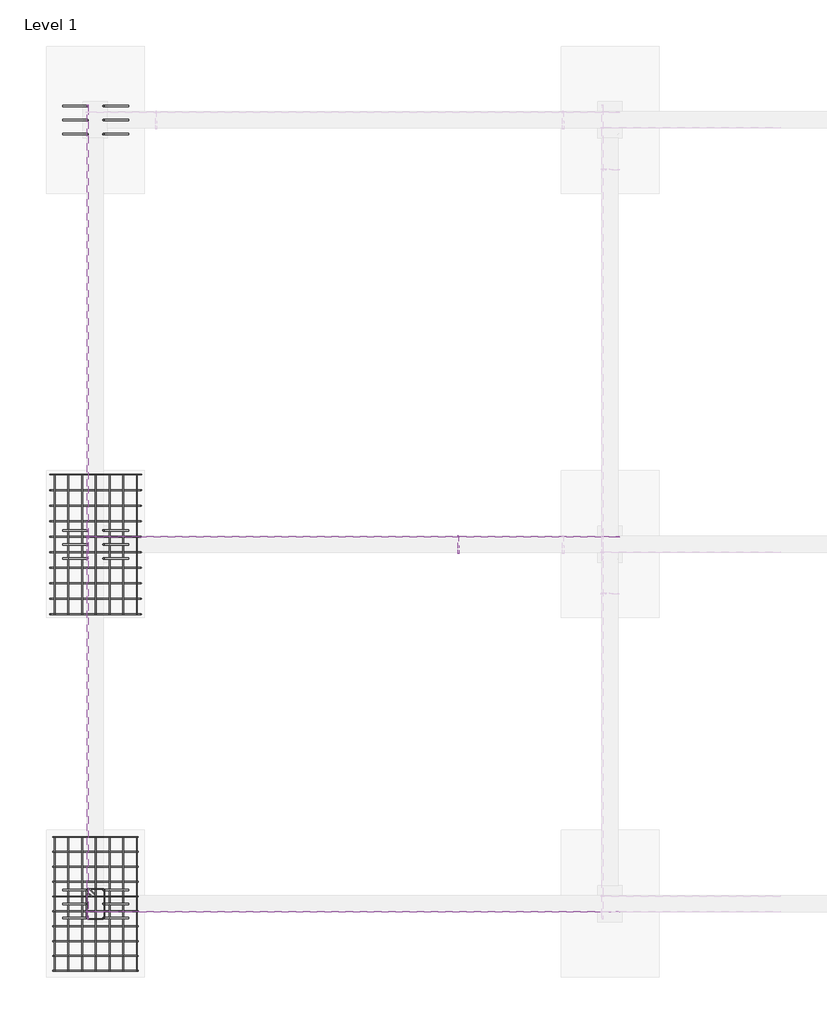
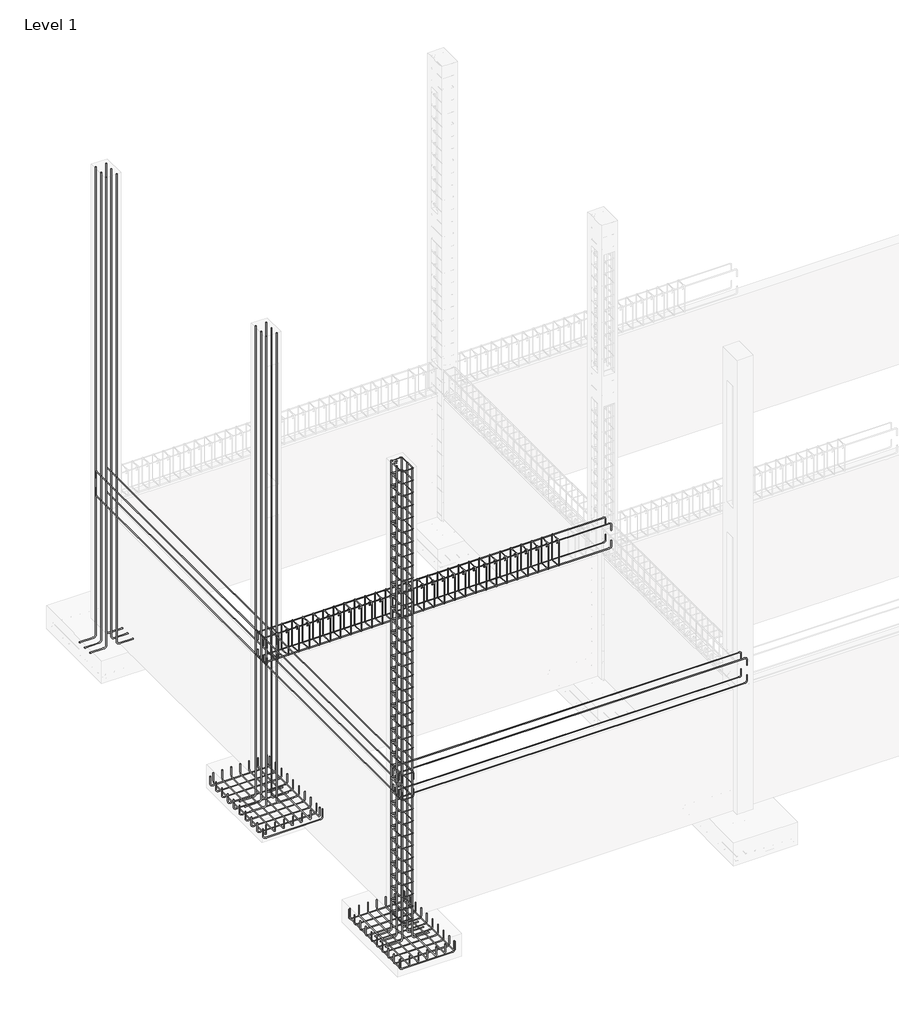
# One storey, part 3 of 8: 20 reinforcing bars.
"""IFC4 building model written with IfcOpenShell, lengths in millimetres."""

from ifc_helpers import new_model, si_unit, point, frame, origin, place, context, project, spatial, polyline, circle_curve, trimmed, segment, composite_curve, source, transform, mapped, element, save
from ifc_brep_helpers import swept_disk

model = new_model("IFC4")

# Units and contexts
model_context = context("Model", 3, world=origin())
ifc_project = project(units=[si_unit("LENGTHUNIT", "METRE", prefix="MILLI")], contexts=[model_context])

# Site, building, storey
site = spatial("IfcSite", under=ifc_project)
building = spatial("IfcBuilding", under=site)
storey = spatial("IfcBuildingStorey", under=building, Name="Level 1", Elevation=0.0)

# Reinforcing bars
placement = place(None, origin())
reinforcing_bar_shape = source(origin(), model_context, "Body", "SolidModel", [
    swept_disk(composite_curve([segment(polyline([(-20238.7033089, 3954.7360327, -178.562), (-20238.7033089, 3954.7360327, -330.962)]), True, "CONTINUOUS"), segment(trimmed(circle_curve(frame((-20282.7723089, 3954.7360327, -330.962), z_axis=(0.0, 1.0, 0.0), x_axis=(44.068999999999505, 0.0, 0.0)), 44.069), [point((-20238.7033089, 3954.7360327, -330.962))], [point((-20282.7723089, 3954.7360327, -375.031))], True, "CARTESIAN"), True, "CONTINUOUS"), segment(polyline([(-20282.7723089, 3954.7360327, -375.031), (-21249.4963089, 3954.7360327, -375.031)]), True, "CONTINUOUS"), segment(trimmed(circle_curve(frame((-21249.4963089, 3954.7360327, -330.962), z_axis=(0.0, 1.0, 0.0), x_axis=(0.0, 0.0, -44.06900000000002)), 44.069), [point((-21249.4963089, 3954.7360327, -375.031))], [point((-21293.5653089, 3954.7360327, -330.962))], True, "CARTESIAN"), True, "CONTINUOUS"), segment(polyline([(-21293.5653089, 3954.7360327, -330.962), (-21293.5653089, 3954.7360327, -178.562)]), True, "CONTINUOUS")], self_intersect=False), 5.969),
])
element("IfcReinforcingBar", 1, at=placement, inside=storey, context=model_context, shape_type="MappedRepresentation", body=[
    mapped(reinforcing_bar_shape, transform((0.0, 0.0, 0.0), x_axis=(1.0, 0.0, 0.0), y_axis=(0.0, 1.0, 0.0), z_axis=(0.0, 0.0, 1.0))),
    mapped(reinforcing_bar_shape, transform((0.0, -184.9402222, 0.0), x_axis=(1.0, 0.0, 0.0), y_axis=(0.0, 1.0, 0.0), z_axis=(0.0, 0.0, 1.0))),
    mapped(reinforcing_bar_shape, transform((0.0, -369.8804444, 0.0), x_axis=(1.0, 0.0, 0.0), y_axis=(0.0, 1.0, 0.0), z_axis=(0.0, 0.0, 1.0))),
    mapped(reinforcing_bar_shape, transform((0.0, -554.8206667, 0.0), x_axis=(1.0, 0.0, 0.0), y_axis=(0.0, 1.0, 0.0), z_axis=(0.0, 0.0, 1.0))),
    mapped(reinforcing_bar_shape, transform((0.0, -739.7608889, 0.0), x_axis=(1.0, 0.0, 0.0), y_axis=(0.0, 1.0, 0.0), z_axis=(0.0, 0.0, 1.0))),
    mapped(reinforcing_bar_shape, transform((0.0, -924.7011111, 0.0), x_axis=(1.0, 0.0, 0.0), y_axis=(0.0, 1.0, 0.0), z_axis=(0.0, 0.0, 1.0))),
    mapped(reinforcing_bar_shape, transform((0.0, -1109.6413333, 0.0), x_axis=(1.0, 0.0, 0.0), y_axis=(0.0, 1.0, 0.0), z_axis=(0.0, 0.0, 1.0))),
    mapped(reinforcing_bar_shape, transform((0.0, -1294.5815556, 0.0), x_axis=(1.0, 0.0, 0.0), y_axis=(0.0, 1.0, 0.0), z_axis=(0.0, 0.0, 1.0))),
    mapped(reinforcing_bar_shape, transform((0.0, -1479.5217778, 0.0), x_axis=(1.0, 0.0, 0.0), y_axis=(0.0, 1.0, 0.0), z_axis=(0.0, 0.0, 1.0))),
    mapped(reinforcing_bar_shape, transform((0.0, -1664.462, 0.0), x_axis=(1.0, 0.0, 0.0), y_axis=(0.0, 1.0, 0.0), z_axis=(0.0, 0.0, 1.0))),
])
reinforcing_bar_2_shape = source(origin(), model_context, "Body", "SolidModel", [
    swept_disk(composite_curve([segment(polyline([(-21274.1343089, 3954.7360327, -165.481), (-21274.1343089, 3954.7360327, -317.881)]), True, "CONTINUOUS"), segment(trimmed(circle_curve(frame((-21274.1343089, 3910.6670327, -317.881), z_axis=(-1.0, 0.0, 0.0), x_axis=(0.0, 44.06899999999996, 0.0)), 44.069), [point((-21274.1343089, 3954.7360327, -317.881))], [point((-21274.1343089, 3910.6670327, -361.95))], True, "CARTESIAN"), True, "CONTINUOUS"), segment(polyline([(-21274.1343089, 3910.6670327, -361.95), (-21274.1343089, 2334.3430327, -361.95)]), True, "CONTINUOUS"), segment(trimmed(circle_curve(frame((-21274.1343089, 2334.3430327, -317.881), z_axis=(-1.0, 0.0, 0.0), x_axis=(0.0, 0.0, -44.06900000000002)), 44.069), [point((-21274.1343089, 2334.3430327, -361.95))], [point((-21274.1343089, 2290.2740327, -317.881))], True, "CARTESIAN"), True, "CONTINUOUS"), segment(polyline([(-21274.1343089, 2290.2740327, -317.881), (-21274.1343089, 2290.2740327, -165.481)]), True, "CONTINUOUS")], self_intersect=False), 5.969),
])
element("IfcReinforcingBar", 2, at=placement, inside=storey, context=model_context, shape_type="MappedRepresentation", body=[
    mapped(reinforcing_bar_2_shape, transform((0.0, 0.0, 0.0), x_axis=(1.0, 0.0, 0.0), y_axis=(0.0, 1.0, 0.0), z_axis=(0.0, 0.0, 1.0))),
    mapped(reinforcing_bar_2_shape, transform((170.5954914, 0.0, 0.0), x_axis=(1.0, 0.0, 0.0), y_axis=(0.0, 1.0, 0.0), z_axis=(0.0, 0.0, 1.0))),
    mapped(reinforcing_bar_2_shape, transform((341.1909829, 0.0, 0.0), x_axis=(1.0, 0.0, 0.0), y_axis=(0.0, 1.0, 0.0), z_axis=(0.0, 0.0, 1.0))),
    mapped(reinforcing_bar_2_shape, transform((511.7864743, 0.0, 0.0), x_axis=(1.0, 0.0, 0.0), y_axis=(0.0, 1.0, 0.0), z_axis=(0.0, 0.0, 1.0))),
    mapped(reinforcing_bar_2_shape, transform((682.3819658, 0.0, 0.0), x_axis=(1.0, 0.0, 0.0), y_axis=(0.0, 1.0, 0.0), z_axis=(0.0, 0.0, 1.0))),
    mapped(reinforcing_bar_2_shape, transform((852.9774572, 0.0, 0.0), x_axis=(1.0, 0.0, 0.0), y_axis=(0.0, 1.0, 0.0), z_axis=(0.0, 0.0, 1.0))),
    mapped(reinforcing_bar_2_shape, transform((1023.5729487, 0.0, 0.0), x_axis=(1.0, 0.0, 0.0), y_axis=(0.0, 1.0, 0.0), z_axis=(0.0, 0.0, 1.0))),
])
reinforcing_bar_3_shape = source(origin(), model_context, "Body", "SolidModel", [
    swept_disk(composite_curve([segment(polyline([(-20667.7093089, 3297.1300327, 9105.9), (-20667.7093089, 3297.1300327, -307.9115)]), True, "CONTINUOUS"), segment(trimmed(circle_curve(frame((-20621.6083089, 3297.1300327, -307.9115), z_axis=(0.0, -1.0, 0.0), x_axis=(-46.10100000000239, 0.0, 0.0)), 46.101), [point((-20667.7093089, 3297.1300327, -307.9115))], [point((-20621.6083089, 3297.1300327, -354.0125))], True, "CARTESIAN"), True, "CONTINUOUS"), segment(polyline([(-20621.6083089, 3297.1300327, -354.0125), (-20355.0353089, 3297.1300327, -354.0125)]), True, "CONTINUOUS")], self_intersect=False), 8.001),
])
element("IfcReinforcingBar", 3, at=placement, inside=storey, context=model_context, shape_type="MappedRepresentation", body=[
    mapped(reinforcing_bar_3_shape, transform((0.0, 0.0, 0.0), x_axis=(1.0, 0.0, 0.0), y_axis=(0.0, 1.0, 0.0), z_axis=(0.0, 0.0, 1.0))),
    mapped(reinforcing_bar_3_shape, transform((0.0, -174.625, 0.0), x_axis=(1.0, 0.0, 0.0), y_axis=(0.0, 1.0, 0.0), z_axis=(0.0, 0.0, 1.0))),
    mapped(reinforcing_bar_3_shape, transform((0.0, -349.25, 0.0), x_axis=(1.0, 0.0, 0.0), y_axis=(0.0, 1.0, 0.0), z_axis=(0.0, 0.0, 1.0))),
])
reinforcing_bar_4_shape = source(origin(), model_context, "Body", "SolidModel", [
    swept_disk(composite_curve([segment(polyline([(-21177.2333089, 3297.1300327, -354.0125), (-20910.6603089, 3297.1300327, -354.0125)]), True, "CONTINUOUS"), segment(trimmed(circle_curve(frame((-20910.6603089, 3297.1300327, -307.9115), z_axis=(0.0, -1.0, 0.0), x_axis=(0.0, 0.0, -46.101)), 46.101), [point((-20910.6603089, 3297.1300327, -354.0125))], [point((-20864.5593089, 3297.1300327, -307.9115))], True, "CARTESIAN"), True, "CONTINUOUS"), segment(polyline([(-20864.5593089, 3297.1300327, -307.9115), (-20864.5593089, 3297.1300327, 9105.9)]), True, "CONTINUOUS")], self_intersect=False), 8.001),
])
element("IfcReinforcingBar", 4, at=placement, inside=storey, context=model_context, shape_type="MappedRepresentation", body=[
    mapped(reinforcing_bar_4_shape, transform((0.0, 0.0, 0.0), x_axis=(1.0, 0.0, 0.0), y_axis=(0.0, 1.0, 0.0), z_axis=(0.0, 0.0, 1.0))),
    mapped(reinforcing_bar_4_shape, transform((0.0, -174.625, 0.0), x_axis=(1.0, 0.0, 0.0), y_axis=(0.0, 1.0, 0.0), z_axis=(0.0, 0.0, 1.0))),
    mapped(reinforcing_bar_4_shape, transform((0.0, -349.25, 0.0), x_axis=(1.0, 0.0, 0.0), y_axis=(0.0, 1.0, 0.0), z_axis=(0.0, 0.0, 1.0))),
])
reinforcing_bar_5_shape = source(origin(), model_context, "Body", "SolidModel", [
    swept_disk(composite_curve([segment(polyline([(-20780.3918482, 3245.4710993, 42.037), (-20837.2560453, 3302.3352963, 42.037)]), True, "CONTINUOUS"), segment(trimmed(circle_curve(frame((-20853.5103089, 3286.0810327, 42.037), z_axis=(0.0, 0.0, 1.0), x_axis=(16.25426359999983, 16.254263600000286, 0.0)), 22.987), [point((-20837.2560453, 3302.3352963, 42.037))], [point((-20876.4973089, 3286.0810327, 42.037))], True, "CARTESIAN"), True, "CONTINUOUS"), segment(polyline([(-20876.4973089, 3286.0810327, 42.037), (-20876.4973089, 2958.9290327, 42.037)]), True, "CONTINUOUS"), segment(trimmed(circle_curve(frame((-20853.5103089, 2958.9290327, 42.037), z_axis=(0.0, 0.0, 1.0), x_axis=(-22.98700000000099, 0.0, 0.0)), 22.987), [point((-20876.4973089, 2958.9290327, 42.037))], [point((-20853.5103089, 2935.9420327, 42.037))], True, "CARTESIAN"), True, "CONTINUOUS"), segment(polyline([(-20853.5103089, 2935.9420327, 42.037), (-20678.7583089, 2935.9420327, 42.037)]), True, "CONTINUOUS"), segment(trimmed(circle_curve(frame((-20678.7583089, 2958.9239161, 41.5520181), z_axis=(0.0, 0.02109809375347505, 0.9997774104469302), x_axis=(0.0, -22.981883400000243, 0.4849819000000011)), 22.987), [point((-20678.7583089, 2935.9420327, 42.037))], [point((-20655.7713089, 2958.9239161, 41.5520181))], True, "CARTESIAN"), True, "CONTINUOUS"), segment(polyline([(-20655.7713089, 2958.9239161, 41.5520181), (-20655.7713089, 3286.0861494, 34.6479819)]), True, "CONTINUOUS"), segment(trimmed(circle_curve(frame((-20678.7583089, 3286.0861494, 34.6479819), z_axis=(0.0, 0.02109809375347505, 0.9997774104469302), x_axis=(22.98700000000099, 0.0, 0.0)), 22.987), [point((-20655.7713089, 3286.0861494, 34.6479819))], [point((-20678.7583089, 3309.0680327, 34.163))], True, "CARTESIAN"), True, "CONTINUOUS"), segment(polyline([(-20678.7583089, 3309.0680327, 34.163), (-20853.5103089, 3309.0680327, 34.163)]), True, "CONTINUOUS"), segment(trimmed(circle_curve(frame((-20853.5103089, 3286.0810327, 34.163), z_axis=(0.0, 0.0, 1.0), x_axis=(0.0, 22.98700000000008, 0.0)), 22.987), [point((-20853.5103089, 3309.0680327, 34.163))], [point((-20869.7645724, 3269.8267692, 34.163))], True, "CARTESIAN"), True, "CONTINUOUS"), segment(polyline([(-20869.7645724, 3269.8267692, 34.163), (-20812.9003754, 3212.9625721, 34.163)]), True, "CONTINUOUS")], self_intersect=False), 3.937),
])
element("IfcReinforcingBar", 5, at=placement, inside=storey, context=model_context, shape_type="MappedRepresentation", body=[
    mapped(reinforcing_bar_5_shape, transform((0.0, 0.0, 0.0), x_axis=(1.0, 0.0, 0.0), y_axis=(0.0, 1.0, 0.0), z_axis=(0.0, 0.0, 1.0))),
    mapped(reinforcing_bar_5_shape, transform((0.0, 0.0, 244.8628649), x_axis=(1.0, 0.0, 0.0), y_axis=(0.0, 1.0, 0.0), z_axis=(0.0, 0.0, 1.0))),
    mapped(reinforcing_bar_5_shape, transform((0.0, 0.0, 489.7257297), x_axis=(1.0, 0.0, 0.0), y_axis=(0.0, 1.0, 0.0), z_axis=(0.0, 0.0, 1.0))),
    mapped(reinforcing_bar_5_shape, transform((0.0, 0.0, 734.5885946), x_axis=(1.0, 0.0, 0.0), y_axis=(0.0, 1.0, 0.0), z_axis=(0.0, 0.0, 1.0))),
    mapped(reinforcing_bar_5_shape, transform((0.0, 0.0, 979.4514595), x_axis=(1.0, 0.0, 0.0), y_axis=(0.0, 1.0, 0.0), z_axis=(0.0, 0.0, 1.0))),
    mapped(reinforcing_bar_5_shape, transform((0.0, 0.0, 1224.3143243), x_axis=(1.0, 0.0, 0.0), y_axis=(0.0, 1.0, 0.0), z_axis=(0.0, 0.0, 1.0))),
    mapped(reinforcing_bar_5_shape, transform((0.0, 0.0, 1469.1771892), x_axis=(1.0, 0.0, 0.0), y_axis=(0.0, 1.0, 0.0), z_axis=(0.0, 0.0, 1.0))),
    mapped(reinforcing_bar_5_shape, transform((0.0, 0.0, 1714.0400541), x_axis=(1.0, 0.0, 0.0), y_axis=(0.0, 1.0, 0.0), z_axis=(0.0, 0.0, 1.0))),
    mapped(reinforcing_bar_5_shape, transform((0.0, 0.0, 1958.9029189), x_axis=(1.0, 0.0, 0.0), y_axis=(0.0, 1.0, 0.0), z_axis=(0.0, 0.0, 1.0))),
    mapped(reinforcing_bar_5_shape, transform((0.0, 0.0, 2203.7657838), x_axis=(1.0, 0.0, 0.0), y_axis=(0.0, 1.0, 0.0), z_axis=(0.0, 0.0, 1.0))),
    mapped(reinforcing_bar_5_shape, transform((0.0, 0.0, 2448.6286486), x_axis=(1.0, 0.0, 0.0), y_axis=(0.0, 1.0, 0.0), z_axis=(0.0, 0.0, 1.0))),
    mapped(reinforcing_bar_5_shape, transform((0.0, 0.0, 2693.4915135), x_axis=(1.0, 0.0, 0.0), y_axis=(0.0, 1.0, 0.0), z_axis=(0.0, 0.0, 1.0))),
    mapped(reinforcing_bar_5_shape, transform((0.0, 0.0, 2938.3543784), x_axis=(1.0, 0.0, 0.0), y_axis=(0.0, 1.0, 0.0), z_axis=(0.0, 0.0, 1.0))),
    mapped(reinforcing_bar_5_shape, transform((0.0, 0.0, 3183.2172432), x_axis=(1.0, 0.0, 0.0), y_axis=(0.0, 1.0, 0.0), z_axis=(0.0, 0.0, 1.0))),
    mapped(reinforcing_bar_5_shape, transform((0.0, 0.0, 3428.0801081), x_axis=(1.0, 0.0, 0.0), y_axis=(0.0, 1.0, 0.0), z_axis=(0.0, 0.0, 1.0))),
    mapped(reinforcing_bar_5_shape, transform((0.0, 0.0, 3672.942973), x_axis=(1.0, 0.0, 0.0), y_axis=(0.0, 1.0, 0.0), z_axis=(0.0, 0.0, 1.0))),
    mapped(reinforcing_bar_5_shape, transform((0.0, 0.0, 3917.8058378), x_axis=(1.0, 0.0, 0.0), y_axis=(0.0, 1.0, 0.0), z_axis=(0.0, 0.0, 1.0))),
    mapped(reinforcing_bar_5_shape, transform((0.0, 0.0, 4162.6687027), x_axis=(1.0, 0.0, 0.0), y_axis=(0.0, 1.0, 0.0), z_axis=(0.0, 0.0, 1.0))),
    mapped(reinforcing_bar_5_shape, transform((0.0, 0.0, 4407.5315676), x_axis=(1.0, 0.0, 0.0), y_axis=(0.0, 1.0, 0.0), z_axis=(0.0, 0.0, 1.0))),
    mapped(reinforcing_bar_5_shape, transform((0.0, 0.0, 4652.3944324), x_axis=(1.0, 0.0, 0.0), y_axis=(0.0, 1.0, 0.0), z_axis=(0.0, 0.0, 1.0))),
    mapped(reinforcing_bar_5_shape, transform((0.0, 0.0, 4897.2572973), x_axis=(1.0, 0.0, 0.0), y_axis=(0.0, 1.0, 0.0), z_axis=(0.0, 0.0, 1.0))),
    mapped(reinforcing_bar_5_shape, transform((0.0, 0.0, 5142.1201622), x_axis=(1.0, 0.0, 0.0), y_axis=(0.0, 1.0, 0.0), z_axis=(0.0, 0.0, 1.0))),
    mapped(reinforcing_bar_5_shape, transform((0.0, 0.0, 5386.983027), x_axis=(1.0, 0.0, 0.0), y_axis=(0.0, 1.0, 0.0), z_axis=(0.0, 0.0, 1.0))),
    mapped(reinforcing_bar_5_shape, transform((0.0, 0.0, 5631.8458919), x_axis=(1.0, 0.0, 0.0), y_axis=(0.0, 1.0, 0.0), z_axis=(0.0, 0.0, 1.0))),
    mapped(reinforcing_bar_5_shape, transform((0.0, 0.0, 5876.7087568), x_axis=(1.0, 0.0, 0.0), y_axis=(0.0, 1.0, 0.0), z_axis=(0.0, 0.0, 1.0))),
    mapped(reinforcing_bar_5_shape, transform((0.0, 0.0, 6121.5716216), x_axis=(1.0, 0.0, 0.0), y_axis=(0.0, 1.0, 0.0), z_axis=(0.0, 0.0, 1.0))),
    mapped(reinforcing_bar_5_shape, transform((0.0, 0.0, 6366.4344865), x_axis=(1.0, 0.0, 0.0), y_axis=(0.0, 1.0, 0.0), z_axis=(0.0, 0.0, 1.0))),
    mapped(reinforcing_bar_5_shape, transform((0.0, 0.0, 6611.2973514), x_axis=(1.0, 0.0, 0.0), y_axis=(0.0, 1.0, 0.0), z_axis=(0.0, 0.0, 1.0))),
    mapped(reinforcing_bar_5_shape, transform((0.0, 0.0, 6856.1602162), x_axis=(1.0, 0.0, 0.0), y_axis=(0.0, 1.0, 0.0), z_axis=(0.0, 0.0, 1.0))),
    mapped(reinforcing_bar_5_shape, transform((0.0, 0.0, 7101.0230811), x_axis=(1.0, 0.0, 0.0), y_axis=(0.0, 1.0, 0.0), z_axis=(0.0, 0.0, 1.0))),
    mapped(reinforcing_bar_5_shape, transform((0.0, 0.0, 7345.8859459), x_axis=(1.0, 0.0, 0.0), y_axis=(0.0, 1.0, 0.0), z_axis=(0.0, 0.0, 1.0))),
    mapped(reinforcing_bar_5_shape, transform((0.0, 0.0, 7590.7488108), x_axis=(1.0, 0.0, 0.0), y_axis=(0.0, 1.0, 0.0), z_axis=(0.0, 0.0, 1.0))),
    mapped(reinforcing_bar_5_shape, transform((0.0, 0.0, 7835.6116757), x_axis=(1.0, 0.0, 0.0), y_axis=(0.0, 1.0, 0.0), z_axis=(0.0, 0.0, 1.0))),
    mapped(reinforcing_bar_5_shape, transform((0.0, 0.0, 8080.4745405), x_axis=(1.0, 0.0, 0.0), y_axis=(0.0, 1.0, 0.0), z_axis=(0.0, 0.0, 1.0))),
    mapped(reinforcing_bar_5_shape, transform((0.0, 0.0, 8325.3374054), x_axis=(1.0, 0.0, 0.0), y_axis=(0.0, 1.0, 0.0), z_axis=(0.0, 0.0, 1.0))),
    mapped(reinforcing_bar_5_shape, transform((0.0, 0.0, 8570.2002703), x_axis=(1.0, 0.0, 0.0), y_axis=(0.0, 1.0, 0.0), z_axis=(0.0, 0.0, 1.0))),
    mapped(reinforcing_bar_5_shape, transform((0.0, 0.0, 8815.0631351), x_axis=(1.0, 0.0, 0.0), y_axis=(0.0, 1.0, 0.0), z_axis=(0.0, 0.0, 1.0))),
    mapped(reinforcing_bar_5_shape, transform((0.0, 0.0, 9059.926), x_axis=(1.0, 0.0, 0.0), y_axis=(0.0, 1.0, 0.0), z_axis=(0.0, 0.0, 1.0))),
])
reinforcing_bar_6_shape = source(origin(), model_context, "Body", "SolidModel", [
    swept_disk(composite_curve([segment(polyline([(-14253.1291545, 3219.1306965, 2643.0183362), (-14253.1291545, 3219.1306965, 2528.7183362)]), True, "CONTINUOUS"), segment(trimmed(circle_curve(frame((-14287.6731545, 3219.1306965, 2528.7183362), z_axis=(0.0, 1.0, 0.0), x_axis=(34.54399999999987, 0.0, 0.0)), 34.544), [point((-14253.1291545, 3219.1306965, 2528.7183362))], [point((-14287.6731545, 3219.1306965, 2494.1743362))], True, "CARTESIAN"), True, "CONTINUOUS"), segment(polyline([(-14287.6731545, 3219.1306965, 2494.1743362), (-20839.9213089, 3219.1306965, 2494.1743362)]), True, "CONTINUOUS"), segment(trimmed(circle_curve(frame((-20839.9213089, 3219.1306965, 2528.7183362), z_axis=(0.0, 1.0, 0.0), x_axis=(0.0, 0.0, -34.54399999999987)), 34.544), [point((-20839.9213089, 3219.1306965, 2494.1743362))], [point((-20874.4653089, 3219.1306965, 2528.7183362))], True, "CARTESIAN"), True, "CONTINUOUS"), segment(polyline([(-20874.4653089, 3219.1306965, 2528.7183362), (-20874.4653089, 3219.1306965, 2643.0183362)]), True, "CONTINUOUS")], self_intersect=False), 5.969),
])
element("IfcReinforcingBar", 6, at=placement, inside=storey, context=model_context, shape_type="MappedRepresentation", body=[
    mapped(reinforcing_bar_6_shape, transform((0.0, 0.0, 0.0), x_axis=(1.0, 0.0, 0.0), y_axis=(0.0, 1.0, 0.0), z_axis=(0.0, 0.0, 1.0))),
    mapped(reinforcing_bar_6_shape, transform((0.0, -193.2513276, 0.0), x_axis=(1.0, 0.0, 0.0), y_axis=(0.0, 1.0, 0.0), z_axis=(0.0, 0.0, 1.0))),
])
reinforcing_bar_7_shape = source(origin(), model_context, "Body", "SolidModel", [
    swept_disk(composite_curve([segment(polyline([(-20874.4653089, 3219.1306965, 2843.3816638), (-20874.4653089, 3219.1306965, 2957.6816638)]), True, "CONTINUOUS"), segment(trimmed(circle_curve(frame((-20839.9213089, 3219.1306965, 2957.6816638), z_axis=(0.0, 1.0, 0.0), x_axis=(-34.54399999999805, 0.0, 0.0)), 34.544), [point((-20874.4653089, 3219.1306965, 2957.6816638))], [point((-20839.9213089, 3219.1306965, 2992.2256638))], True, "CARTESIAN"), True, "CONTINUOUS"), segment(polyline([(-20839.9213089, 3219.1306965, 2992.2256638), (-14287.6731545, 3219.1306965, 2992.2256638)]), True, "CONTINUOUS"), segment(trimmed(circle_curve(frame((-14287.6731545, 3219.1306965, 2957.6816638), z_axis=(0.0, 1.0, 0.0), x_axis=(0.0, 0.0, 34.54399999999987)), 34.544), [point((-14287.6731545, 3219.1306965, 2992.2256638))], [point((-14253.1291545, 3219.1306965, 2957.6816638))], True, "CARTESIAN"), True, "CONTINUOUS"), segment(polyline([(-14253.1291545, 3219.1306965, 2957.6816638), (-14253.1291545, 3219.1306965, 2843.3816638)]), True, "CONTINUOUS")], self_intersect=False), 5.969),
])
element("IfcReinforcingBar", 7, at=placement, inside=storey, context=model_context, shape_type="MappedRepresentation", body=[
    mapped(reinforcing_bar_7_shape, transform((0.0, 0.0, 0.0), x_axis=(1.0, 0.0, 0.0), y_axis=(0.0, 1.0, 0.0), z_axis=(0.0, 0.0, 1.0))),
    mapped(reinforcing_bar_7_shape, transform((0.0, -193.2513276, 0.0), x_axis=(1.0, 0.0, 0.0), y_axis=(0.0, 1.0, 0.0), z_axis=(0.0, 0.0, 1.0))),
])
reinforcing_bar_8_shape = source(origin(), model_context, "Body", "SolidModel", [
    swept_disk(composite_curve([segment(polyline([(-20667.7093089, 13046.2805262, 9105.9), (-20667.7093089, 13046.2805262, -307.9115)]), True, "CONTINUOUS"), segment(trimmed(circle_curve(frame((-20621.6083089, 13046.2805262, -307.9115), z_axis=(0.0, -1.0, 0.0), x_axis=(-46.10100000000239, 0.0, 0.0)), 46.101), [point((-20667.7093089, 13046.2805262, -307.9115))], [point((-20621.6083089, 13046.2805262, -354.0125))], True, "CARTESIAN"), True, "CONTINUOUS"), segment(polyline([(-20621.6083089, 13046.2805262, -354.0125), (-20355.0353089, 13046.2805262, -354.0125)]), True, "CONTINUOUS")], self_intersect=False), 8.001),
])
element("IfcReinforcingBar", 8, at=placement, inside=storey, context=model_context, shape_type="MappedRepresentation", body=[
    mapped(reinforcing_bar_8_shape, transform((0.0, 0.0, 0.0), x_axis=(1.0, 0.0, 0.0), y_axis=(0.0, 1.0, 0.0), z_axis=(0.0, 0.0, 1.0))),
    mapped(reinforcing_bar_8_shape, transform((0.0, -174.625, 0.0), x_axis=(1.0, 0.0, 0.0), y_axis=(0.0, 1.0, 0.0), z_axis=(0.0, 0.0, 1.0))),
    mapped(reinforcing_bar_8_shape, transform((0.0, -349.25, 0.0), x_axis=(1.0, 0.0, 0.0), y_axis=(0.0, 1.0, 0.0), z_axis=(0.0, 0.0, 1.0))),
])
reinforcing_bar_9_shape = source(origin(), model_context, "Body", "SolidModel", [
    swept_disk(composite_curve([segment(polyline([(-21177.2333089, 13046.2805262, -354.0125), (-20910.6603089, 13046.2805262, -354.0125)]), True, "CONTINUOUS"), segment(trimmed(circle_curve(frame((-20910.6603089, 13046.2805262, -307.9115), z_axis=(0.0, -1.0, 0.0), x_axis=(0.0, 0.0, -46.101)), 46.101), [point((-20910.6603089, 13046.2805262, -354.0125))], [point((-20864.5593089, 13046.2805262, -307.9115))], True, "CARTESIAN"), True, "CONTINUOUS"), segment(polyline([(-20864.5593089, 13046.2805262, -307.9115), (-20864.5593089, 13046.2805262, 9105.9)]), True, "CONTINUOUS")], self_intersect=False), 8.001),
])
element("IfcReinforcingBar", 9, at=placement, inside=storey, context=model_context, shape_type="MappedRepresentation", body=[
    mapped(reinforcing_bar_9_shape, transform((0.0, 0.0, 0.0), x_axis=(1.0, 0.0, 0.0), y_axis=(0.0, 1.0, 0.0), z_axis=(0.0, 0.0, 1.0))),
    mapped(reinforcing_bar_9_shape, transform((0.0, -174.625, 0.0), x_axis=(1.0, 0.0, 0.0), y_axis=(0.0, 1.0, 0.0), z_axis=(0.0, 0.0, 1.0))),
    mapped(reinforcing_bar_9_shape, transform((0.0, -349.25, 0.0), x_axis=(1.0, 0.0, 0.0), y_axis=(0.0, 1.0, 0.0), z_axis=(0.0, 0.0, 1.0))),
])
reinforcing_bar_10_shape = source(origin(), model_context, "Body", "SolidModel", [
    swept_disk(composite_curve([segment(polyline([(-20667.7093089, 7767.9070829, 9105.9), (-20667.7093089, 7767.9070829, -307.9115)]), True, "CONTINUOUS"), segment(trimmed(circle_curve(frame((-20621.6083089, 7767.9070829, -307.9115), z_axis=(0.0, -1.0, 0.0), x_axis=(-46.10100000000239, 0.0, 0.0)), 46.101), [point((-20667.7093089, 7767.9070829, -307.9115))], [point((-20621.6083089, 7767.9070829, -354.0125))], True, "CARTESIAN"), True, "CONTINUOUS"), segment(polyline([(-20621.6083089, 7767.9070829, -354.0125), (-20355.0353089, 7767.9070829, -354.0125)]), True, "CONTINUOUS")], self_intersect=False), 8.001),
])
element("IfcReinforcingBar", 10, at=placement, inside=storey, context=model_context, shape_type="MappedRepresentation", body=[
    mapped(reinforcing_bar_10_shape, transform((0.0, 0.0, 0.0), x_axis=(1.0, 0.0, 0.0), y_axis=(0.0, 1.0, 0.0), z_axis=(0.0, 0.0, 1.0))),
    mapped(reinforcing_bar_10_shape, transform((0.0, -174.625, 0.0), x_axis=(1.0, 0.0, 0.0), y_axis=(0.0, 1.0, 0.0), z_axis=(0.0, 0.0, 1.0))),
    mapped(reinforcing_bar_10_shape, transform((0.0, -349.25, 0.0), x_axis=(1.0, 0.0, 0.0), y_axis=(0.0, 1.0, 0.0), z_axis=(0.0, 0.0, 1.0))),
])
reinforcing_bar_11_shape = source(origin(), model_context, "Body", "SolidModel", [
    swept_disk(composite_curve([segment(polyline([(-21177.2333089, 7767.9070829, -354.0125), (-20910.6603089, 7767.9070829, -354.0125)]), True, "CONTINUOUS"), segment(trimmed(circle_curve(frame((-20910.6603089, 7767.9070829, -307.9115), z_axis=(0.0, -1.0, 0.0), x_axis=(0.0, 0.0, -46.101)), 46.101), [point((-20910.6603089, 7767.9070829, -354.0125))], [point((-20864.5593089, 7767.9070829, -307.9115))], True, "CARTESIAN"), True, "CONTINUOUS"), segment(polyline([(-20864.5593089, 7767.9070829, -307.9115), (-20864.5593089, 7767.9070829, 9105.9)]), True, "CONTINUOUS")], self_intersect=False), 8.001),
])
element("IfcReinforcingBar", 11, at=placement, inside=storey, context=model_context, shape_type="MappedRepresentation", body=[
    mapped(reinforcing_bar_11_shape, transform((0.0, 0.0, 0.0), x_axis=(1.0, 0.0, 0.0), y_axis=(0.0, 1.0, 0.0), z_axis=(0.0, 0.0, 1.0))),
    mapped(reinforcing_bar_11_shape, transform((0.0, -174.625, 0.0), x_axis=(1.0, 0.0, 0.0), y_axis=(0.0, 1.0, 0.0), z_axis=(0.0, 0.0, 1.0))),
    mapped(reinforcing_bar_11_shape, transform((0.0, -349.25, 0.0), x_axis=(1.0, 0.0, 0.0), y_axis=(0.0, 1.0, 0.0), z_axis=(0.0, 0.0, 1.0))),
])
reinforcing_bar_12_shape = source(origin(), model_context, "Body", "SolidModel", [
    swept_disk(composite_curve([segment(polyline([(-20200.6033089, 8463.6130829, -216.662), (-20200.6033089, 8463.6130829, -369.062)]), True, "CONTINUOUS"), segment(trimmed(circle_curve(frame((-20244.6723089, 8463.6130829, -369.062), z_axis=(0.0, 1.0, 0.0), x_axis=(44.068999999999505, 0.0, 0.0)), 44.069), [point((-20200.6033089, 8463.6130829, -369.062))], [point((-20244.6723089, 8463.6130829, -413.131))], True, "CARTESIAN"), True, "CONTINUOUS"), segment(polyline([(-20244.6723089, 8463.6130829, -413.131), (-21287.5963089, 8463.6130829, -413.131)]), True, "CONTINUOUS"), segment(trimmed(circle_curve(frame((-21287.5963089, 8463.6130829, -369.062), z_axis=(0.0, 1.0, 0.0), x_axis=(0.0, 0.0, -44.06899999999996)), 44.069), [point((-21287.5963089, 8463.6130829, -413.131))], [point((-21331.6653089, 8463.6130829, -369.062))], True, "CARTESIAN"), True, "CONTINUOUS"), segment(polyline([(-21331.6653089, 8463.6130829, -369.062), (-21331.6653089, 8463.6130829, -216.662)]), True, "CONTINUOUS")], self_intersect=False), 5.969),
])
element("IfcReinforcingBar", 12, at=placement, inside=storey, context=model_context, shape_type="MappedRepresentation", body=[
    mapped(reinforcing_bar_12_shape, transform((0.0, 0.0, 0.0), x_axis=(1.0, 0.0, 0.0), y_axis=(0.0, 1.0, 0.0), z_axis=(0.0, 0.0, 1.0))),
    mapped(reinforcing_bar_12_shape, transform((0.0, -193.4068889, 0.0), x_axis=(1.0, 0.0, 0.0), y_axis=(0.0, 1.0, 0.0), z_axis=(0.0, 0.0, 1.0))),
    mapped(reinforcing_bar_12_shape, transform((0.0, -386.8137778, 0.0), x_axis=(1.0, 0.0, 0.0), y_axis=(0.0, 1.0, 0.0), z_axis=(0.0, 0.0, 1.0))),
    mapped(reinforcing_bar_12_shape, transform((0.0, -580.2206667, 0.0), x_axis=(1.0, 0.0, 0.0), y_axis=(0.0, 1.0, 0.0), z_axis=(0.0, 0.0, 1.0))),
    mapped(reinforcing_bar_12_shape, transform((0.0, -773.6275556, 0.0), x_axis=(1.0, 0.0, 0.0), y_axis=(0.0, 1.0, 0.0), z_axis=(0.0, 0.0, 1.0))),
    mapped(reinforcing_bar_12_shape, transform((0.0, -967.0344444, 0.0), x_axis=(1.0, 0.0, 0.0), y_axis=(0.0, 1.0, 0.0), z_axis=(0.0, 0.0, 1.0))),
    mapped(reinforcing_bar_12_shape, transform((0.0, -1160.4413333, 0.0), x_axis=(1.0, 0.0, 0.0), y_axis=(0.0, 1.0, 0.0), z_axis=(0.0, 0.0, 1.0))),
    mapped(reinforcing_bar_12_shape, transform((0.0, -1353.8482222, 0.0), x_axis=(1.0, 0.0, 0.0), y_axis=(0.0, 1.0, 0.0), z_axis=(0.0, 0.0, 1.0))),
    mapped(reinforcing_bar_12_shape, transform((0.0, -1547.2551111, 0.0), x_axis=(1.0, 0.0, 0.0), y_axis=(0.0, 1.0, 0.0), z_axis=(0.0, 0.0, 1.0))),
    mapped(reinforcing_bar_12_shape, transform((0.0, -1740.662, 0.0), x_axis=(1.0, 0.0, 0.0), y_axis=(0.0, 1.0, 0.0), z_axis=(0.0, 0.0, 1.0))),
])
reinforcing_bar_13_shape = source(origin(), model_context, "Body", "SolidModel", [
    swept_disk(composite_curve([segment(polyline([(-21274.1343089, 8463.6130829, -165.481), (-21274.1343089, 8463.6130829, -317.881)]), True, "CONTINUOUS"), segment(trimmed(circle_curve(frame((-21274.1343089, 8419.5440829, -317.881), z_axis=(-1.0, 0.0, 0.0), x_axis=(0.0, 44.068999999999505, 0.0)), 44.069), [point((-21274.1343089, 8463.6130829, -317.881))], [point((-21274.1343089, 8419.5440829, -361.95))], True, "CARTESIAN"), True, "CONTINUOUS"), segment(polyline([(-21274.1343089, 8419.5440829, -361.95), (-21274.1343089, 6767.0200829, -361.95)]), True, "CONTINUOUS"), segment(trimmed(circle_curve(frame((-21274.1343089, 6767.0200829, -317.881), z_axis=(-1.0, 0.0, 0.0), x_axis=(0.0, 0.0, -44.06900000000002)), 44.069), [point((-21274.1343089, 6767.0200829, -361.95))], [point((-21274.1343089, 6722.9510829, -317.881))], True, "CARTESIAN"), True, "CONTINUOUS"), segment(polyline([(-21274.1343089, 6722.9510829, -317.881), (-21274.1343089, 6722.9510829, -165.481)]), True, "CONTINUOUS")], self_intersect=False), 5.969),
])
element("IfcReinforcingBar", 13, at=placement, inside=storey, context=model_context, shape_type="MappedRepresentation", body=[
    mapped(reinforcing_bar_13_shape, transform((0.0, 0.0, 0.0), x_axis=(1.0, 0.0, 0.0), y_axis=(0.0, 1.0, 0.0), z_axis=(0.0, 0.0, 1.0))),
    mapped(reinforcing_bar_13_shape, transform((170.5954914, 0.0, 0.0), x_axis=(1.0, 0.0, 0.0), y_axis=(0.0, 1.0, 0.0), z_axis=(0.0, 0.0, 1.0))),
    mapped(reinforcing_bar_13_shape, transform((341.1909829, 0.0, 0.0), x_axis=(1.0, 0.0, 0.0), y_axis=(0.0, 1.0, 0.0), z_axis=(0.0, 0.0, 1.0))),
    mapped(reinforcing_bar_13_shape, transform((511.7864743, 0.0, 0.0), x_axis=(1.0, 0.0, 0.0), y_axis=(0.0, 1.0, 0.0), z_axis=(0.0, 0.0, 1.0))),
    mapped(reinforcing_bar_13_shape, transform((682.3819658, 0.0, 0.0), x_axis=(1.0, 0.0, 0.0), y_axis=(0.0, 1.0, 0.0), z_axis=(0.0, 0.0, 1.0))),
    mapped(reinforcing_bar_13_shape, transform((852.9774572, 0.0, 0.0), x_axis=(1.0, 0.0, 0.0), y_axis=(0.0, 1.0, 0.0), z_axis=(0.0, 0.0, 1.0))),
    mapped(reinforcing_bar_13_shape, transform((1023.5729487, 0.0, 0.0), x_axis=(1.0, 0.0, 0.0), y_axis=(0.0, 1.0, 0.0), z_axis=(0.0, 0.0, 1.0))),
])
reinforcing_bar_14_shape = source(origin(), model_context, "Body", "SolidModel", [
    swept_disk(composite_curve([segment(polyline([(-20874.4653089, 7496.6564191, 2643.0183362), (-20874.4653089, 7496.6564191, 2528.7183362)]), True, "CONTINUOUS"), segment(trimmed(circle_curve(frame((-20839.9213089, 7496.6564191, 2528.7183362), z_axis=(0.0, -1.0, 0.0), x_axis=(-34.54399999999805, 0.0, 0.0)), 34.544), [point((-20874.4653089, 7496.6564191, 2528.7183362))], [point((-20839.9213089, 7496.6564191, 2494.1743362))], True, "CARTESIAN"), True, "CONTINUOUS"), segment(polyline([(-20839.9213089, 7496.6564191, 2494.1743362), (-14287.6731545, 7496.6564191, 2494.1743362)]), True, "CONTINUOUS"), segment(trimmed(circle_curve(frame((-14287.6731545, 7496.6564191, 2528.7183362), z_axis=(0.0, -1.0, 0.0), x_axis=(0.0, 0.0, -34.54399999999987)), 34.544), [point((-14287.6731545, 7496.6564191, 2494.1743362))], [point((-14253.1291545, 7496.6564191, 2528.7183362))], True, "CARTESIAN"), True, "CONTINUOUS"), segment(polyline([(-14253.1291545, 7496.6564191, 2528.7183362), (-14253.1291545, 7496.6564191, 2643.0183362)]), True, "CONTINUOUS")], self_intersect=False), 5.969),
])
element("IfcReinforcingBar", 14, at=placement, inside=storey, context=model_context, shape_type="MappedRepresentation", body=[
    mapped(reinforcing_bar_14_shape, transform((0.0, 0.0, 0.0), x_axis=(1.0, 0.0, 0.0), y_axis=(0.0, 1.0, 0.0), z_axis=(0.0, 0.0, 1.0))),
    mapped(reinforcing_bar_14_shape, transform((0.0, 193.2513276, 0.0), x_axis=(1.0, 0.0, 0.0), y_axis=(0.0, 1.0, 0.0), z_axis=(0.0, 0.0, 1.0))),
])
reinforcing_bar_15_shape = source(origin(), model_context, "Body", "SolidModel", [
    swept_disk(composite_curve([segment(polyline([(-14253.1291545, 7496.6564191, 2843.3816638), (-14253.1291545, 7496.6564191, 2957.6816638)]), True, "CONTINUOUS"), segment(trimmed(circle_curve(frame((-14287.6731545, 7496.6564191, 2957.6816638), z_axis=(0.0, -1.0, 0.0), x_axis=(34.54399999999987, 0.0, 0.0)), 34.544), [point((-14253.1291545, 7496.6564191, 2957.6816638))], [point((-14287.6731545, 7496.6564191, 2992.2256638))], True, "CARTESIAN"), True, "CONTINUOUS"), segment(polyline([(-14287.6731545, 7496.6564191, 2992.2256638), (-20839.9213089, 7496.6564191, 2992.2256638)]), True, "CONTINUOUS"), segment(trimmed(circle_curve(frame((-20839.9213089, 7496.6564191, 2957.6816638), z_axis=(0.0, -1.0, 0.0), x_axis=(0.0, 0.0, 34.54399999999987)), 34.544), [point((-20839.9213089, 7496.6564191, 2992.2256638))], [point((-20874.4653089, 7496.6564191, 2957.6816638))], True, "CARTESIAN"), True, "CONTINUOUS"), segment(polyline([(-20874.4653089, 7496.6564191, 2957.6816638), (-20874.4653089, 7496.6564191, 2843.3816638)]), True, "CONTINUOUS")], self_intersect=False), 5.969),
])
element("IfcReinforcingBar", 15, at=placement, inside=storey, context=model_context, shape_type="MappedRepresentation", body=[
    mapped(reinforcing_bar_15_shape, transform((0.0, 0.0, 0.0), x_axis=(1.0, 0.0, 0.0), y_axis=(0.0, 1.0, 0.0), z_axis=(0.0, 0.0, 1.0))),
    mapped(reinforcing_bar_15_shape, transform((0.0, 193.2513276, 0.0), x_axis=(1.0, 0.0, 0.0), y_axis=(0.0, 1.0, 0.0), z_axis=(0.0, 0.0, 1.0))),
])
reinforcing_bar_16_shape = source(origin(), model_context, "Body", "SolidModel", [
    swept_disk(composite_curve([segment(polyline([(-15262.6578092, 7546.5160164, 2909.8575394), (-15262.6578092, 7489.6518193, 2966.7217364)]), True, "CONTINUOUS"), segment(trimmed(circle_curve(frame((-15262.6578092, 7505.9060829, 2982.976), z_axis=(-1.0, 0.0, 0.0), x_axis=(0.0, -16.25426359999983, -16.254263600000286)), 22.987), [point((-15262.6578092, 7489.6518193, 2966.7217364))], [point((-15262.6578092, 7505.9060829, 3005.963))], True, "CARTESIAN"), True, "CONTINUOUS"), segment(polyline([(-15262.6578092, 7505.9060829, 3005.963), (-15262.6578092, 7680.6580829, 3005.963)]), True, "CONTINUOUS"), segment(trimmed(circle_curve(frame((-15262.6578092, 7680.6580829, 2982.976), z_axis=(-1.0, 0.0, 0.0), x_axis=(0.0, 0.0, 22.98700000000008)), 22.987), [point((-15262.6578092, 7680.6580829, 3005.963))], [point((-15262.6578092, 7703.6450829, 2982.976))], True, "CARTESIAN"), True, "CONTINUOUS"), segment(polyline([(-15262.6578092, 7703.6450829, 2982.976), (-15262.6578092, 7703.6450829, 2503.424)]), True, "CONTINUOUS"), segment(trimmed(circle_curve(frame((-15261.8383109, 7680.6726953, 2503.424), z_axis=(-0.9993643184948482, -0.03565051078634927, 0.0), x_axis=(-0.8194982999993954, 22.97238759999982, 0.0)), 22.987), [point((-15262.6578092, 7703.6450829, 2503.424))], [point((-15261.8383109, 7680.6726953, 2480.437))], True, "CARTESIAN"), True, "CONTINUOUS"), segment(polyline([(-15261.8383109, 7680.6726953, 2480.437), (-15255.6033075, 7505.8914705, 2480.437)]), True, "CONTINUOUS"), segment(trimmed(circle_curve(frame((-15255.6033075, 7505.8914705, 2503.424), z_axis=(-0.9993643184948482, -0.03565051078634927, 0.0), x_axis=(0.0, 0.0, -22.98700000000008)), 22.987), [point((-15255.6033075, 7505.8914705, 2480.437))], [point((-15254.7838092, 7482.9190829, 2503.424))], True, "CARTESIAN"), True, "CONTINUOUS"), segment(polyline([(-15254.7838092, 7482.9190829, 2503.424), (-15254.7838092, 7482.9190829, 2982.976)]), True, "CONTINUOUS"), segment(trimmed(circle_curve(frame((-15254.7838092, 7505.9060829, 2982.976), z_axis=(-1.0, 0.0, 0.0), x_axis=(0.0, -22.98700000000008, 0.0)), 22.987), [point((-15254.7838092, 7482.9190829, 2982.976))], [point((-15254.7838092, 7522.1603465, 2999.2302636))], True, "CARTESIAN"), True, "CONTINUOUS"), segment(polyline([(-15254.7838092, 7522.1603465, 2999.2302636), (-15254.7838092, 7579.0245435, 2942.3660665)]), True, "CONTINUOUS")], self_intersect=False), 3.937),
])
element("IfcReinforcingBar", 16, at=placement, inside=storey, context=model_context, shape_type="MappedRepresentation", body=[
    mapped(reinforcing_bar_16_shape, transform((0.0, 0.0, 0.0), x_axis=(1.0, 0.0, 0.0), y_axis=(0.0, 1.0, 0.0), z_axis=(0.0, 0.0, 1.0))),
    mapped(reinforcing_bar_16_shape, transform((-198.0422037, 0.0, 0.0), x_axis=(1.0, 0.0, 0.0), y_axis=(0.0, 1.0, 0.0), z_axis=(0.0, 0.0, 1.0))),
    mapped(reinforcing_bar_16_shape, transform((-396.0844074, 0.0, 0.0), x_axis=(1.0, 0.0, 0.0), y_axis=(0.0, 1.0, 0.0), z_axis=(0.0, 0.0, 1.0))),
    mapped(reinforcing_bar_16_shape, transform((-594.1266111, 0.0, 0.0), x_axis=(1.0, 0.0, 0.0), y_axis=(0.0, 1.0, 0.0), z_axis=(0.0, 0.0, 1.0))),
    mapped(reinforcing_bar_16_shape, transform((-792.1688148, 0.0, 0.0), x_axis=(1.0, 0.0, 0.0), y_axis=(0.0, 1.0, 0.0), z_axis=(0.0, 0.0, 1.0))),
    mapped(reinforcing_bar_16_shape, transform((-990.2110185, 0.0, 0.0), x_axis=(1.0, 0.0, 0.0), y_axis=(0.0, 1.0, 0.0), z_axis=(0.0, 0.0, 1.0))),
    mapped(reinforcing_bar_16_shape, transform((-1188.2532221, 0.0, 0.0), x_axis=(1.0, 0.0, 0.0), y_axis=(0.0, 1.0, 0.0), z_axis=(0.0, 0.0, 1.0))),
    mapped(reinforcing_bar_16_shape, transform((-1386.2954258, 0.0, 0.0), x_axis=(1.0, 0.0, 0.0), y_axis=(0.0, 1.0, 0.0), z_axis=(0.0, 0.0, 1.0))),
    mapped(reinforcing_bar_16_shape, transform((-1584.3376295, 0.0, 0.0), x_axis=(1.0, 0.0, 0.0), y_axis=(0.0, 1.0, 0.0), z_axis=(0.0, 0.0, 1.0))),
    mapped(reinforcing_bar_16_shape, transform((-1782.3798332, 0.0, 0.0), x_axis=(1.0, 0.0, 0.0), y_axis=(0.0, 1.0, 0.0), z_axis=(0.0, 0.0, 1.0))),
    mapped(reinforcing_bar_16_shape, transform((-1980.4220369, 0.0, 0.0), x_axis=(1.0, 0.0, 0.0), y_axis=(0.0, 1.0, 0.0), z_axis=(0.0, 0.0, 1.0))),
    mapped(reinforcing_bar_16_shape, transform((-2178.4642406, 0.0, 0.0), x_axis=(1.0, 0.0, 0.0), y_axis=(0.0, 1.0, 0.0), z_axis=(0.0, 0.0, 1.0))),
    mapped(reinforcing_bar_16_shape, transform((-2376.5064443, 0.0, 0.0), x_axis=(1.0, 0.0, 0.0), y_axis=(0.0, 1.0, 0.0), z_axis=(0.0, 0.0, 1.0))),
    mapped(reinforcing_bar_16_shape, transform((-2574.548648, 0.0, 0.0), x_axis=(1.0, 0.0, 0.0), y_axis=(0.0, 1.0, 0.0), z_axis=(0.0, 0.0, 1.0))),
    mapped(reinforcing_bar_16_shape, transform((-2772.5908517, 0.0, 0.0), x_axis=(1.0, 0.0, 0.0), y_axis=(0.0, 1.0, 0.0), z_axis=(0.0, 0.0, 1.0))),
    mapped(reinforcing_bar_16_shape, transform((-2970.6330554, 0.0, 0.0), x_axis=(1.0, 0.0, 0.0), y_axis=(0.0, 1.0, 0.0), z_axis=(0.0, 0.0, 1.0))),
    mapped(reinforcing_bar_16_shape, transform((-3168.6752591, 0.0, 0.0), x_axis=(1.0, 0.0, 0.0), y_axis=(0.0, 1.0, 0.0), z_axis=(0.0, 0.0, 1.0))),
    mapped(reinforcing_bar_16_shape, transform((-3366.7174628, 0.0, 0.0), x_axis=(1.0, 0.0, 0.0), y_axis=(0.0, 1.0, 0.0), z_axis=(0.0, 0.0, 1.0))),
    mapped(reinforcing_bar_16_shape, transform((-3564.7596664, 0.0, 0.0), x_axis=(1.0, 0.0, 0.0), y_axis=(0.0, 1.0, 0.0), z_axis=(0.0, 0.0, 1.0))),
    mapped(reinforcing_bar_16_shape, transform((-3762.8018701, 0.0, 0.0), x_axis=(1.0, 0.0, 0.0), y_axis=(0.0, 1.0, 0.0), z_axis=(0.0, 0.0, 1.0))),
    mapped(reinforcing_bar_16_shape, transform((-3960.8440738, 0.0, 0.0), x_axis=(1.0, 0.0, 0.0), y_axis=(0.0, 1.0, 0.0), z_axis=(0.0, 0.0, 1.0))),
    mapped(reinforcing_bar_16_shape, transform((-4158.8862775, 0.0, 0.0), x_axis=(1.0, 0.0, 0.0), y_axis=(0.0, 1.0, 0.0), z_axis=(0.0, 0.0, 1.0))),
    mapped(reinforcing_bar_16_shape, transform((-4356.9284812, 0.0, 0.0), x_axis=(1.0, 0.0, 0.0), y_axis=(0.0, 1.0, 0.0), z_axis=(0.0, 0.0, 1.0))),
    mapped(reinforcing_bar_16_shape, transform((-4554.9706849, 0.0, 0.0), x_axis=(1.0, 0.0, 0.0), y_axis=(0.0, 1.0, 0.0), z_axis=(0.0, 0.0, 1.0))),
    mapped(reinforcing_bar_16_shape, transform((-4753.0128886, 0.0, 0.0), x_axis=(1.0, 0.0, 0.0), y_axis=(0.0, 1.0, 0.0), z_axis=(0.0, 0.0, 1.0))),
    mapped(reinforcing_bar_16_shape, transform((-4951.0550923, 0.0, 0.0), x_axis=(1.0, 0.0, 0.0), y_axis=(0.0, 1.0, 0.0), z_axis=(0.0, 0.0, 1.0))),
    mapped(reinforcing_bar_16_shape, transform((-5149.097296, 0.0, 0.0), x_axis=(1.0, 0.0, 0.0), y_axis=(0.0, 1.0, 0.0), z_axis=(0.0, 0.0, 1.0))),
    mapped(reinforcing_bar_16_shape, transform((-5347.1394997, 0.0, 0.0), x_axis=(1.0, 0.0, 0.0), y_axis=(0.0, 1.0, 0.0), z_axis=(0.0, 0.0, 1.0))),
])
reinforcing_bar_17_shape = source(origin(), model_context, "Body", "SolidModel", [
    swept_disk(composite_curve([segment(polyline([(-20862.7599727, 7777.8130829, 2643.0183362), (-20862.7599727, 7777.8130829, 2528.7183362)]), True, "CONTINUOUS"), segment(trimmed(circle_curve(frame((-20862.7599727, 7743.2690829, 2528.7183362), z_axis=(-1.0, 0.0, 0.0), x_axis=(0.0, 34.54399999999987, 0.0)), 34.544), [point((-20862.7599727, 7777.8130829, 2528.7183362))], [point((-20862.7599727, 7743.2690829, 2494.1743362))], True, "CARTESIAN"), True, "CONTINUOUS"), segment(polyline([(-20862.7599727, 7743.2690829, 2494.1743362), (-20862.7599727, 2972.5180327, 2494.1743362)]), True, "CONTINUOUS"), segment(trimmed(circle_curve(frame((-20862.7599727, 2972.5180327, 2528.7183362), z_axis=(-1.0, 0.0, 0.0), x_axis=(0.0, 0.0, -34.54399999999987)), 34.544), [point((-20862.7599727, 2972.5180327, 2494.1743362))], [point((-20862.7599727, 2937.9740327, 2528.7183362))], True, "CARTESIAN"), True, "CONTINUOUS"), segment(polyline([(-20862.7599727, 2937.9740327, 2528.7183362), (-20862.7599727, 2937.9740327, 2643.0183362)]), True, "CONTINUOUS")], self_intersect=False), 5.969),
])
element("IfcReinforcingBar", 17, at=placement, inside=storey, context=model_context, shape_type="MappedRepresentation", body=[
    mapped(reinforcing_bar_17_shape, transform((0.0, 0.0, 0.0), x_axis=(1.0, 0.0, 0.0), y_axis=(0.0, 1.0, 0.0), z_axis=(0.0, 0.0, 1.0))),
    mapped(reinforcing_bar_17_shape, transform((204.9566638, 0.0, 0.0), x_axis=(1.0, 0.0, 0.0), y_axis=(0.0, 1.0, 0.0), z_axis=(0.0, 0.0, 1.0))),
])
reinforcing_bar_18_shape = source(origin(), model_context, "Body", "SolidModel", [
    swept_disk(composite_curve([segment(polyline([(-20862.7599727, 2937.9740327, 2843.3816638), (-20862.7599727, 2937.9740327, 2957.6816638)]), True, "CONTINUOUS"), segment(trimmed(circle_curve(frame((-20862.7599727, 2972.5180327, 2957.6816638), z_axis=(-1.0, 0.0, 0.0), x_axis=(0.0, -34.54399999999987, 0.0)), 34.544), [point((-20862.7599727, 2937.9740327, 2957.6816638))], [point((-20862.7599727, 2972.5180327, 2992.2256638))], True, "CARTESIAN"), True, "CONTINUOUS"), segment(polyline([(-20862.7599727, 2972.5180327, 2992.2256638), (-20862.7599727, 7743.2690829, 2992.2256638)]), True, "CONTINUOUS"), segment(trimmed(circle_curve(frame((-20862.7599727, 7743.2690829, 2957.6816638), z_axis=(-1.0, 0.0, 0.0), x_axis=(0.0, 0.0, 34.54399999999987)), 34.544), [point((-20862.7599727, 7743.2690829, 2992.2256638))], [point((-20862.7599727, 7777.8130829, 2957.6816638))], True, "CARTESIAN"), True, "CONTINUOUS"), segment(polyline([(-20862.7599727, 7777.8130829, 2957.6816638), (-20862.7599727, 7777.8130829, 2843.3816638)]), True, "CONTINUOUS")], self_intersect=False), 5.969),
])
element("IfcReinforcingBar", 18, at=placement, inside=storey, context=model_context, shape_type="MappedRepresentation", body=[
    mapped(reinforcing_bar_18_shape, transform((0.0, 0.0, 0.0), x_axis=(1.0, 0.0, 0.0), y_axis=(0.0, 1.0, 0.0), z_axis=(0.0, 0.0, 1.0))),
    mapped(reinforcing_bar_18_shape, transform((204.9566638, 0.0, 0.0), x_axis=(1.0, 0.0, 0.0), y_axis=(0.0, 1.0, 0.0), z_axis=(0.0, 0.0, 1.0))),
])
reinforcing_bar_19_shape = source(origin(), model_context, "Body", "SolidModel", [
    swept_disk(composite_curve([segment(polyline([(-20862.7599727, 13056.1865262, 2643.0183362), (-20862.7599727, 13056.1865262, 2528.7183362)]), True, "CONTINUOUS"), segment(trimmed(circle_curve(frame((-20862.7599727, 13021.6425262, 2528.7183362), z_axis=(-1.0, 0.0, 0.0), x_axis=(0.0, 34.54399999999987, 0.0)), 34.544), [point((-20862.7599727, 13056.1865262, 2528.7183362))], [point((-20862.7599727, 13021.6425262, 2494.1743362))], True, "CARTESIAN"), True, "CONTINUOUS"), segment(polyline([(-20862.7599727, 13021.6425262, 2494.1743362), (-20862.7599727, 7443.2950829, 2494.1743362)]), True, "CONTINUOUS"), segment(trimmed(circle_curve(frame((-20862.7599727, 7443.2950829, 2528.7183362), z_axis=(-1.0, 0.0, 0.0), x_axis=(0.0, 0.0, -34.54399999999987)), 34.544), [point((-20862.7599727, 7443.2950829, 2494.1743362))], [point((-20862.7599727, 7408.7510829, 2528.7183362))], True, "CARTESIAN"), True, "CONTINUOUS"), segment(polyline([(-20862.7599727, 7408.7510829, 2528.7183362), (-20862.7599727, 7408.7510829, 2643.0183362)]), True, "CONTINUOUS")], self_intersect=False), 5.969),
])
element("IfcReinforcingBar", 19, at=placement, inside=storey, context=model_context, shape_type="MappedRepresentation", body=[
    mapped(reinforcing_bar_19_shape, transform((0.0, 0.0, 0.0), x_axis=(1.0, 0.0, 0.0), y_axis=(0.0, 1.0, 0.0), z_axis=(0.0, 0.0, 1.0))),
    mapped(reinforcing_bar_19_shape, transform((204.9566638, 0.0, 0.0), x_axis=(1.0, 0.0, 0.0), y_axis=(0.0, 1.0, 0.0), z_axis=(0.0, 0.0, 1.0))),
])
reinforcing_bar_20_shape = source(origin(), model_context, "Body", "SolidModel", [
    swept_disk(composite_curve([segment(polyline([(-20862.7599727, 7408.7510829, 2843.3816638), (-20862.7599727, 7408.7510829, 2957.6816638)]), True, "CONTINUOUS"), segment(trimmed(circle_curve(frame((-20862.7599727, 7443.2950829, 2957.6816638), z_axis=(-1.0, 0.0, 0.0), x_axis=(0.0, -34.54399999999987, 0.0)), 34.544), [point((-20862.7599727, 7408.7510829, 2957.6816638))], [point((-20862.7599727, 7443.2950829, 2992.2256638))], True, "CARTESIAN"), True, "CONTINUOUS"), segment(polyline([(-20862.7599727, 7443.2950829, 2992.2256638), (-20862.7599727, 13021.6425262, 2992.2256638)]), True, "CONTINUOUS"), segment(trimmed(circle_curve(frame((-20862.7599727, 13021.6425262, 2957.6816638), z_axis=(-1.0, 0.0, 0.0), x_axis=(0.0, 0.0, 34.54399999999987)), 34.544), [point((-20862.7599727, 13021.6425262, 2992.2256638))], [point((-20862.7599727, 13056.1865262, 2957.6816638))], True, "CARTESIAN"), True, "CONTINUOUS"), segment(polyline([(-20862.7599727, 13056.1865262, 2957.6816638), (-20862.7599727, 13056.1865262, 2843.3816638)]), True, "CONTINUOUS")], self_intersect=False), 5.969),
])
element("IfcReinforcingBar", 20, at=placement, inside=storey, context=model_context, shape_type="MappedRepresentation", body=[
    mapped(reinforcing_bar_20_shape, transform((0.0, 0.0, 0.0), x_axis=(1.0, 0.0, 0.0), y_axis=(0.0, 1.0, 0.0), z_axis=(0.0, 0.0, 1.0))),
    mapped(reinforcing_bar_20_shape, transform((204.9566638, 0.0, 0.0), x_axis=(1.0, 0.0, 0.0), y_axis=(0.0, 1.0, 0.0), z_axis=(0.0, 0.0, 1.0))),
])

save(model, "model.ifc")

# Revit data of these elements
# Elements 1, 2, 3, 4, 5, 6, 7, 8, 9, 10, 11, 12, 13, 14, 15, 16, 17, 18, 19, 20 (IfcReinforcingBar)
#   Phase Created = New Construction
